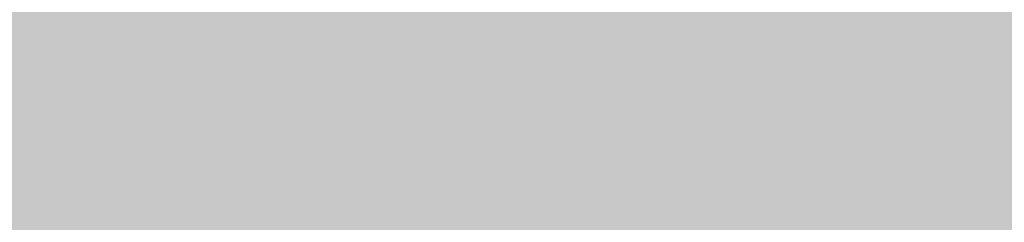
# Model space of a CAD drawing. Units: feet. Extents: x 3168 to 4724, y 827 to 1477.
# Tile 204 of 256: x 3333 to 3364, y 1087 to 1094. Entities that reach past the tile are written whole.
import ezdxf

# ---------------------------------------------------------------- set-up
doc = ezdxf.new("R2010")
doc.units = ezdxf.units.FT
doc.layers.add('A-ELEV-PATT', color=8, linetype='Continuous', lineweight=13)

msp = doc.modelspace()

# ---------------------------------------------------------------- hatches: boundary and pattern name
at = {"layer": 'A-ELEV-PATT'}
h = msp.add_hatch(color=256, dxfattribs=at)
h.dxf.hatch_style = 1
edge = h.paths.add_edge_path()
edge.add_ellipse((3552.906, 979.22), major_axis=(36.745, 0), ratio=0.484848, start_angle=0, end_angle=360)
edge = h.paths.add_edge_path()
edge.add_ellipse((3559.892, 929.252), major_axis=(36.745, 0), ratio=0.484848, start_angle=0, end_angle=360)
edge = h.paths.add_edge_path()
edge.add_line((3299.317, 1198.606), (3479.917, 1198.606))
edge.add_line((3479.917, 1198.606), (3479.917, 1209.869))
edge.add_spline(control_points=[(3479.917, 1209.869), (3464.301, 1209.869), (3448.686, 1209.869), (3410.949, 1209.869), (3388.828, 1209.869), (3355.647, 1209.869), (3344.586, 1209.869), (3327.996, 1209.869), (3322.466, 1209.869), (3314.17, 1209.869), (3311.405, 1209.869), (3307.257, 1209.869), (3305.875, 1209.869), (3303.801, 1209.869), (3303.11, 1209.869), (3302.073, 1209.869), (3301.727, 1209.869), (3301.209, 1209.869), (3301.036, 1209.869), (3300.777, 1209.869), (3300.69, 1209.869), (3300.561, 1209.869), (3300.517, 1209.869), (3300.453, 1209.869), (3300.431, 1209.869), (3300.399, 1209.869), (3300.388, 1209.869), (3300.366, 1209.869), (3300.346, 1209.869), (3300.346, 1209.869), (3300.346, 1209.869), (3300.343, 1209.869), (3300.341, 1209.869), (3300.338, 1209.869), (3300.337, 1209.869), (3300.334, 1209.869), (3300.332, 1209.869), (3300.326, 1209.869), (3300.321, 1209.869), (3300.311, 1209.869), (3300.306, 1209.869), (3300.291, 1209.869), (3300.28, 1209.869), (3300.232, 1209.869), (3300.195, 1209.869), (3299.951, 1209.871), (3299.745, 1209.874), (3299.437, 1209.883), (3299.334, 1209.887), (3299.181, 1209.893), (3299.13, 1209.895), (3298.652, 1209.917), (3298.229, 1209.946), (3297.602, 1210.002), (3297.393, 1210.023), (3297.083, 1210.058), (3296.979, 1210.07), (3296.293, 1210.155), (3295.718, 1210.243), (3294.869, 1210.399), (3294.588, 1210.454), (3294.169, 1210.543), (3294.03, 1210.574), (3291.707, 1211.101), (3289.654, 1211.813), (3285.776, 1213.564), (3283.951, 1214.603), (3280.512, 1216.98), (3278.897, 1218.318), (3276.38, 1220.829), (3275.416, 1221.918), (3274.039, 1223.708), (3273.581, 1224.35), (3273.143, 1225.016)], knot_values=[39.119033, 39.119033, 39.119033, 39.119033, 39.286353, 39.286353, 39.523379, 39.523379, 39.641892, 39.641892, 39.701148, 39.701148, 39.730777, 39.730777, 39.745591, 39.745591, 39.752998, 39.752998, 39.756701, 39.756701, 39.758553, 39.758553, 39.759479, 39.759479, 39.759942, 39.759942, 39.760173, 39.760173, 39.760289, 39.760289, 39.760405, 39.760405, 39.760463, 39.760463, 39.763389, 39.763389, 39.764851, 39.764851, 39.767304, 39.767304, 39.773825, 39.773825, 39.78057, 39.78057, 39.79477, 39.79477, 39.845194, 39.845194, 40.126715, 40.126715, 40.267476, 40.267476, 40.337856, 40.337856, 40.927023, 40.927023, 41.221606, 41.221606, 41.368898, 41.368898, 42.202622, 42.202622, 42.619485, 42.619485, 42.827916, 42.827916, 46.118323, 46.118323, 49.408731, 49.408731, 52.699139, 52.699139, 54.927489, 54.927489, 56.104228, 56.104228, 56.104228, 56.104228], weights=[1, 1, 1, 1, 1, 1, 1, 1, 1, 1, 1, 1, 1, 1, 1, 1, 1, 1, 1, 1, 1, 1, 1, 1, 1, 1, 1, 1, 1, 1, 1, 1, 1, 1, 1, 1, 1, 1, 1, 1, 1, 1, 1, 1, 1, 1, 1, 1, 1, 1, 1, 1, 1, 1, 1, 1, 1, 1, 1, 1, 1, 1, 1, 1, 1, 1, 1, 1, 1, 1, 1, 1, 1, 1], degree=3, periodic=0)
edge.add_line((3273.143, 1225.016), (3273.143, 1099.016))
edge.add_line((3273.143, 1099.016), (3299.317, 1099.016))
edge.add_line((3299.317, 1099.016), (3299.317, 1198.606))
edge = h.paths.add_edge_path()
edge.add_line((3304.758, 1324.158), (3479.917, 1324.158))
edge.add_line((3479.917, 1324.158), (3479.917, 1335.715))
edge.add_line((3479.917, 1335.715), (3269.162, 1335.715))
edge.add_spline(control_points=[(3269.162, 1335.715), (3264.024, 1335.715), (3258.364, 1328.958), (3259.264, 1323.9)], knot_values=[0, 0, 0, 0, 15.412191, 15.412191, 15.412191, 15.412191], degree=3, periodic=0)
edge.add_line((3259.264, 1323.9), (3265.517, 1288.769))
edge.add_line((3265.517, 1288.769), (3275.265, 1261.546))
edge.add_line((3275.265, 1261.546), (3304.758, 1261.546))
edge.add_line((3304.758, 1261.546), (3304.758, 1324.158))
h = msp.add_hatch(color=256, dxfattribs=at)
h.dxf.hatch_style = 1
h.paths.add_polyline_path([(3384.525, 1099.016), (3335.029, 1099.016), (3299.317, 1099.016), (3273.143, 1099.016), (3217.565, 1099.016), (3168.069, 827.116), (3335.029, 827.116)])

doc.saveas('drawing.dxf')
